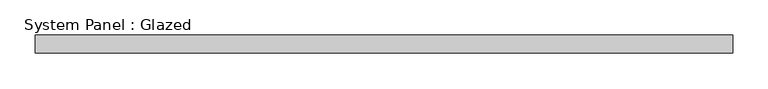
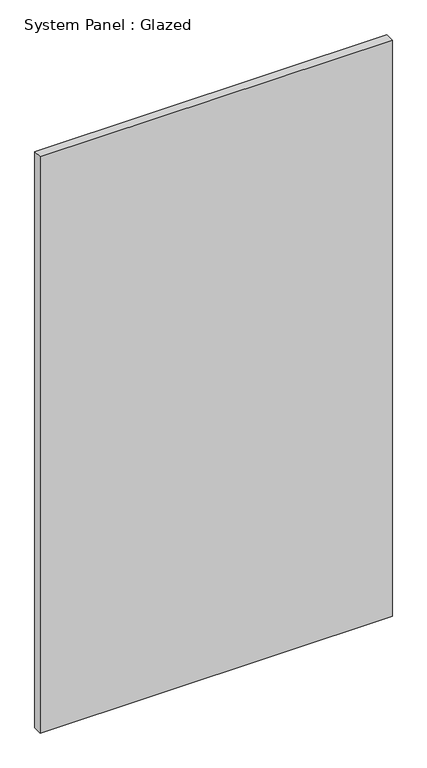
"""IFC4 building model written with IfcOpenShell, lengths in millimetres: plate geometry, System Panel : Glazed."""

from ifc_helpers import new_model, si_unit, origin, origin_with_axes, place, context, project, spatial, polyline, outline, extrude, source, transform, mapped, element, save


def system_panel_glazed_5745033b(model_context):
    return source(origin(), model_context, "Body", "SweptSolid", [
        extrude(outline(polyline([(492.125, 19.05), (-492.125, 19.05), (-492.125, 44.45), (492.125, 44.45), (492.125, 19.05)])), origin_with_axes(), (0.0, 0.0, 1.0), 1701.8),
    ])


if __name__ == "__main__":
    model = new_model("IFC4")
    model_context = context("Model", 3, world=origin())
    ifc_project = project(units=[si_unit("LENGTHUNIT", "METRE", prefix="MILLI")], contexts=[model_context])
    site = spatial("IfcSite", under=ifc_project)
    building = spatial("IfcBuilding", under=site)
    placement = place(None, origin())
    system_panel_glazed_shape = system_panel_glazed_5745033b(model_context)
    element("IfcPlate", 1, ObjectType="System Panel : Glazed", at=placement, inside=building, context=model_context, shape_type="MappedRepresentation", body=[
        mapped(system_panel_glazed_shape, transform((0.0, 0.0, 0.0), x_axis=(1.0, 0.0, 0.0), y_axis=(0.0, 1.0, 0.0), z_axis=(0.0, 0.0, 1.0))),
    ])
    save(model, "model.ifc")

# Revit data of these elements
# Type "System Panel : Glazed"
#   Construction Type Id = "GSP4R"
#   Analytic Construction = "1/8 in Pilkington single glazing"
#   Visual Light Transmittance = 0.9
#   Solar Heat Gain Coefficient = 0.86
#   Heat Transfer Coefficient (U) = 1.18115 BTU/(h·ft²·°F)
# Element 1 (IfcPlate, "System Panel : Glazed")
#   Materials on its faces: "Glass"
# Materials
#   "Glass": class "Glass", colour RGB 0 128 192, transparency 0.75, Description = "Soda Lime Glass", Cost = 0
